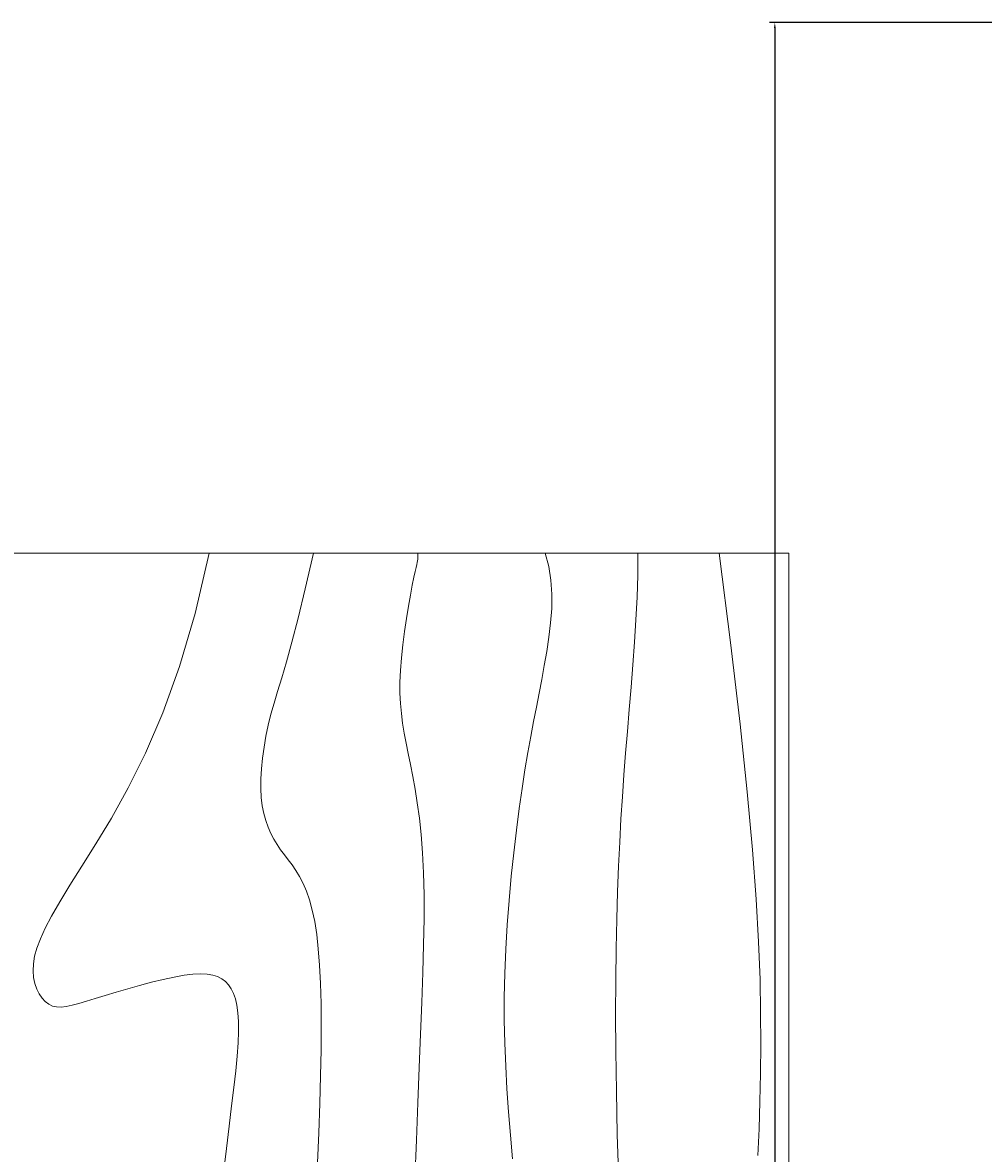
# Model space of a CAD drawing. Units: inches. Extents: x -301 to 715, y -607 to 364.
# Tile 109 of 141: x 43 to 77, y 107 to 146. Entities that reach past the tile are written whole.
import ezdxf

# ---------------------------------------------------------------- set-up
doc = ezdxf.new("R2010")
doc.units = ezdxf.units.IN
doc.header["$MEASUREMENT"] = 0
doc.layers.add('A-ANNO-DIMS', color=2, linetype='Continuous', lineweight=18)
doc.layers.add('A-FURN', color=8, linetype='Continuous', lineweight=18)
doc.styles.get("Standard").update_dxf_attribs({"font": 'arial.ttf'})
doc.dimstyles.get("Standard").update_dxf_attribs({"dimtxt": 0.18, "dimasz": 0.18, "dimexe": 0.18, "dimexo": 0.0625, "dimgap": 0.09, "dimtad": 0, "dimtih": 1, "dimtoh": 1, "dimdec": 1, "dimzin": 0, "dimdsep": 46, "dimlunit": 4, "dimtxsty": 'Standard', "dimcen": 0.09, "dimclrd": 3, "dimclre": 4, "dimclrt": 6, "dimadec": 0, "dimazin": 0, "dimtfac": 1, "dimtdec": 1, "dimtofl": 0, "dimtmove": 0, "dimatfit": 3, "dimfxl": 1, "dimtfill": 2, "dimtfillclr": 51, "dimtolj": 1, "dimtzin": 0, "dimarcsym": 0})

# ---------------------------------------------------------------- blocks, each defined once
blk = doc.blocks.new('Table - Rectangular Woodgrain 60 x 30 in.')
for p, q in [((60, -30), (60, 0)), ((0, -30), (60, -30))]:
    blk.add_line(p, q)
for points in [[(38.6129, -10.4996), (39.4531, -10.5969), (40.223, -10.6895), (40.925, -10.775), (41.5613, -10.8512), (42.1344, -10.9156), (42.6465, -10.966), (43.1, -11), (43.4976, -11.0158), (43.8437, -11.0136), (44.143, -10.9942), (44.4, -10.9583), (44.6195, -10.9069), (44.8062, -10.8406), (44.9648, -10.7603), (45.1, -10.6667), (45.2155, -10.5598), (45.3114, -10.4365), (45.3871, -10.2929), (45.4416, -10.125), (45.4743, -9.929), (45.4844, -9.7011), (45.4709, -9.4371), (45.4333, -9.1333), (45.3716, -8.7883), (45.2896, -8.4104), (45.1919, -8.0107), (45.0833, -7.6), (44.9685, -7.1893), (44.8521, -6.7896), (44.7388, -6.4117), (44.6333, -6.0667), (44.54, -5.7628), (44.4614, -5.4979), (44.4001, -5.2675), (44.3583, -5.0667), (44.3384, -4.8909), (44.3427, -4.7354), (44.3736, -4.5956), (44.4333, -4.4667), (44.5236, -4.3453), (44.6427, -4.2333), (44.7884, -4.1339), (44.9583, -4.05), (45.1501, -3.9849), (45.3614, -3.9417), (45.59, -3.9234), (45.8333, -3.9333), (46.0915, -3.9749), (46.3734, -4.0531), (46.6906, -4.1736), (47.0542, -4.3417), (47.4756, -4.5629), (47.9661, -4.8427), (48.5372, -5.1866), (49.2, -5.6), (49.9676, -6.0844), (50.8594, -6.625), (51.8965, -7.2031), (53.1, -7.8), (54.491, -8.3969), (56.0906, -8.975), (57.9199, -9.5156), (60, -10)], [(38.9578, -13.743), (40, -13.7833), (41.0047, -13.8174), (41.9625, -13.8438), (42.864, -13.8607), (43.7, -13.8667), (44.4631, -13.8604), (45.1552, -13.8417), (45.7801, -13.8104), (46.3416, -13.7667), (46.8439, -13.7104), (47.2906, -13.6417), (47.6858, -13.5604), (48.0333, -13.4667), (48.3375, -13.3608), (48.6042, -13.2448), (48.8396, -13.121), (49.05, -12.9917), (49.2417, -12.8593), (49.4208, -12.7261), (49.5937, -12.5944), (49.7667, -12.4667), (49.9452, -12.3451), (50.1323, -12.2313), (50.3303, -12.1268), (50.5416, -12.0333), (50.7686, -11.9524), (51.0135, -11.8854), (51.2788, -11.8341), (51.5666, -11.8), (51.8785, -11.7843), (52.2116, -11.7865), (52.562, -11.8059), (52.926, -11.8417), (53.2998, -11.8931), (53.6795, -11.9594), (54.0614, -12.0397), (54.4416, -12.1333), (54.8223, -12.2401), (55.2293, -12.3625), (55.6942, -12.5037), (56.2489, -12.6667), (56.9251, -12.8547), (57.7545, -13.0708), (58.7689, -13.3182), (60, -13.6)], [(38.3906, -17.1026), (39.7499, -17.1503), (41.0333, -17.2), (42.2519, -17.2496), (43.4073, -17.2969), (44.4986, -17.3395), (45.525, -17.375), (46.4858, -17.4012), (47.3802, -17.4156), (48.2074, -17.416), (48.9667, -17.4), (49.6583, -17.3662), (50.2872, -17.3167), (50.8595, -17.2547), (51.3812, -17.1833), (51.8584, -17.1057), (52.2971, -17.025), (52.7034, -16.9443), (53.0833, -16.8667), (53.443, -16.7951), (53.789, -16.7313), (54.128, -16.6768), (54.4666, -16.6334), (54.8115, -16.6024), (55.1693, -16.5854), (55.5465, -16.5841), (55.95, -16.6), (56.3828, -16.6337), (56.8346, -16.6823), (57.2915, -16.7418), (57.7396, -16.8084), (58.165, -16.878), (58.5539, -16.9469), (58.8924, -17.0111), (59.1666, -17.0667), (59.3679, -17.1107), (59.5078, -17.1438), (59.6032, -17.1675), (59.6708, -17.1833), (59.7275, -17.193), (59.7901, -17.1979), (59.8753, -17.1998), (60, -17.2)], [(39.1, -20.4667), (39.9164, -20.3951), (40.7187, -20.3313), (41.5117, -20.2768), (42.3, -20.2333), (43.0883, -20.2024), (43.8812, -20.1854), (44.6836, -20.1841), (45.5, -20.2), (46.3328, -20.234), (47.1747, -20.2844), (48.0163, -20.3488), (48.8479, -20.425), (49.66, -20.5106), (50.4429, -20.6031), (51.1872, -20.7004), (51.8833, -20.8), (52.5246, -20.8999), (53.1166, -20.9995), (53.6681, -21.0983), (54.1875, -21.1958), (54.6834, -21.2919), (55.1646, -21.3859), (55.6394, -21.4777), (56.1167, -21.5667), (56.6028, -21.6515), (57.0961, -21.7266), (57.5929, -21.7852), (58.0896, -21.8208), (58.5823, -21.8268), (59.0674, -21.7964), (59.5412, -21.723), (60, -21.6)], [(38.3213, -24.1341), (39.9417, -24.0854), (41.437, -24.0523), (42.8167, -24.0333), (44.0901, -24.0268), (45.2667, -24.0313), (46.3557, -24.0451), (47.3667, -24.0667), (48.309, -24.0947), (49.1928, -24.1287), (50.0284, -24.168), (50.826, -24.2125), (51.5959, -24.2617), (52.3483, -24.3151), (53.0935, -24.3725), (53.8417, -24.4334), (54.6009, -24.497), (55.3699, -24.561), (56.1454, -24.6226), (56.9239, -24.6792), (57.7021, -24.7279), (58.4764, -24.7662), (59.2435, -24.7911), (60, -24.8)], [(39.2137, -28.9412), (40.1375, -28.9792), (41.0753, -29.0093), (42.0432, -29.0297), (43.0572, -29.0384), (44.1333, -29.0333), (45.2936, -29.0114), (46.5843, -28.9641), (48.0579, -28.8816), (49.7666, -28.7542), (51.7629, -28.5721), (54.0989, -28.3255), (56.8272, -28.0048), (60, -27.6)]]:
    blk.add_lwpolyline(points)
blk = doc.blocks.new('*D132')
at = {"layer": 'A-ANNO-DIMS', "color": 4, "lineweight": -2, "transparency": 16777216}
for p, q in [((83.224, 145.954), (69.239, 145.954)), ((83.224, 53.504), (69.239, 53.504))]:
    blk.add_line(p, q, dxfattribs=at)
at = {"layer": 'A-ANNO-DIMS', "color": 3, "lineweight": -2, "transparency": 16777216}
for p, q in [((69.419, 145.774), (69.419, 99.912)), ((69.419, 53.684), (69.419, 99.546))]:
    blk.add_line(p, q, dxfattribs=at)
at = {"layer": 'A-ANNO-DIMS', "color": 3, "transparency": 16777216}
for points in [[(69.389, 145.774), (69.449, 145.774), (69.419, 145.954)], [(69.389, 53.684), (69.449, 53.684), (69.419, 53.504)]]:
    blk.add_solid(points, dxfattribs=at)
at = {"layer": 'Defpoints', "color": 0, "transparency": 16777216}
for p in [(83.287, 145.954), (69.419, 53.504), (83.287, 53.504)]:
    blk.add_point(p, dxfattribs=at)
at = {"layer": 'A-ANNO-DIMS', "color": 6, "transparency": 16777216, "insert": (69.419, 99.729), "char_height": 0.18, "attachment_point": 5, "bg_fill": 1, "box_fill_scale": 1.25, "bg_fill_color": 51, "bg_fill_transparency": 0}
blk.add_mtext('\\A1;SOFA 7\'-8 1/2"', dxfattribs=at)

msp = doc.modelspace()

# ---------------------------------------------------------------- block references
at = {"layer": 'A-FURN', "rotation": 90}
msp.add_blockref('Table - Rectangular Woodgrain 60 x 30 in.', (39.897, 67.651), dxfattribs=at)

# ---------------------------------------------------------------- dimensions: what is measured, and where the dimension line sits
at = {"layer": 'A-ANNO-DIMS'}
dim = msp.add_linear_dim(base=(69.4192, 53.5044), p1=(83.2867, 145.9543), p2=(83.2867, 53.5044), angle=270, text='SOFA <>', dimstyle='Standard', override={"dimdec": 1, "dimlfac": 1, "dimrnd": 0, "dimzin": 1, "dimdsep": 46, "dimlunit": 4, "dimfrac": 2}, dxfattribs=at)
dim.commit()
dim.dimension.update_dxf_attribs({"geometry": '*D132', "text_midpoint": (69.4192, 99.7293)})

doc.saveas('drawing.dxf')
